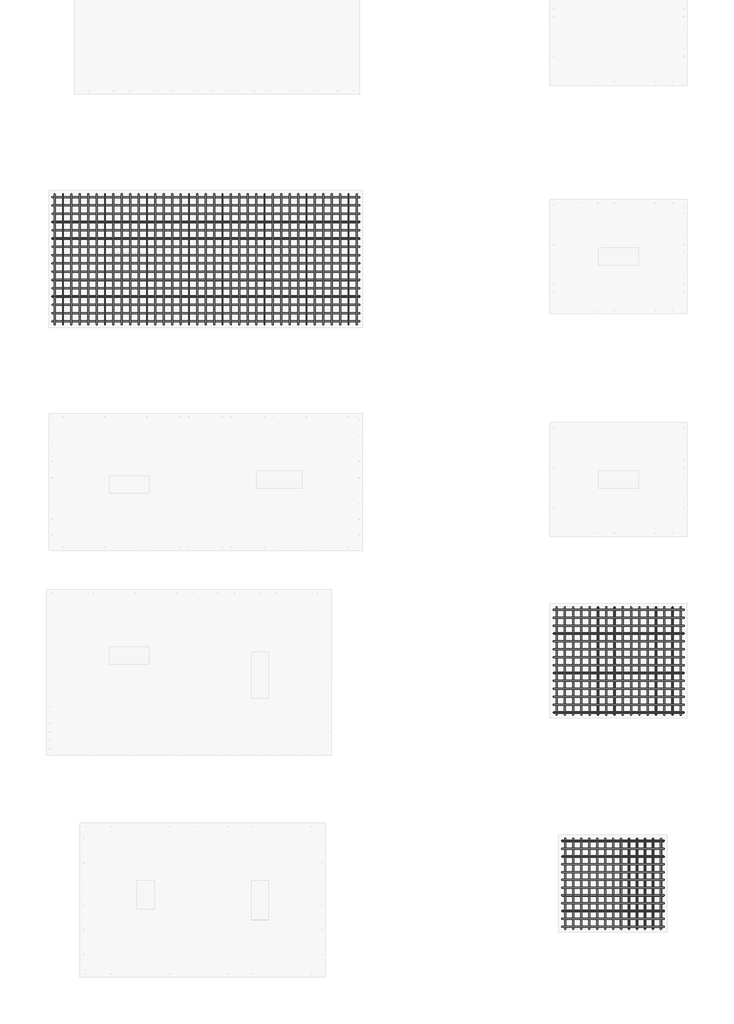
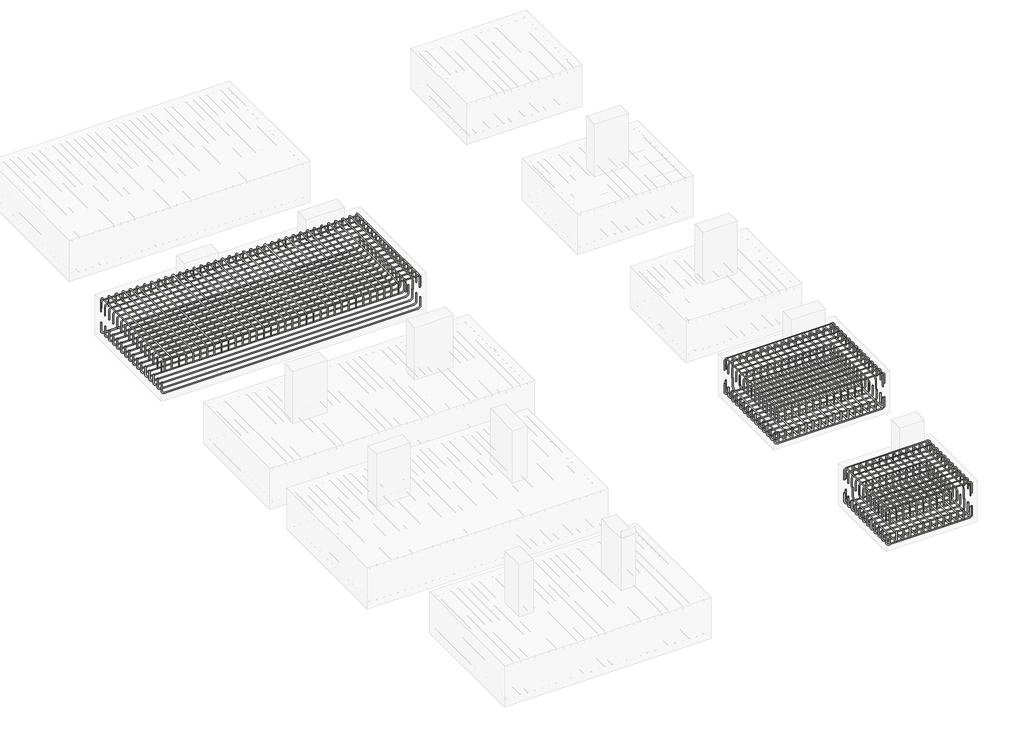
# One storey, part 8 of 21: 11 reinforcing bars.
"""IFC4 building model written with IfcOpenShell, lengths in millimetres."""

from ifc_helpers import new_model, si_unit, point, frame, origin, place, context, project, spatial, polyline, circle_curve, trimmed, segment, composite_curve, source, transform, mapped, element, save
from ifc_brep_helpers import swept_disk

model = new_model("IFC4")

# Units and contexts
model_context = context("Model", 3, world=origin())
ifc_project = project(units=[si_unit("LENGTHUNIT", "METRE", prefix="MILLI")], contexts=[model_context])

# Site, building, storey
site = spatial("IfcSite", under=ifc_project)
building = spatial("IfcBuilding", under=site)
storey = spatial("IfcBuildingStorey", under=building, Elevation=-1100.0)

# Reinforcing bars
placement = place(None, origin())
reinforcing_bar_shape = source(origin(), model_context, "Body", "SolidModel", [
    swept_disk(composite_curve([segment(polyline([(10485.4160849, -1642.8795712, -1400.0), (10485.4160849, -1642.8795712, -1213.4)]), True, "CONTINUOUS"), segment(trimmed(circle_curve(frame((10485.4160849, -1587.4295712, -1213.4), z_axis=(-1.0, 0.0, 0.0), x_axis=(0.0, -55.450000000000045, 0.0)), 55.45), [point((10485.4160849, -1642.8795712, -1213.4))], [point((10485.4160849, -1587.4295712, -1157.95))], True, "CARTESIAN"), True, "CONTINUOUS"), segment(polyline([(10485.4160849, -1587.4295712, -1157.95), (10485.4160849, 585.7704288, -1157.95)]), True, "CONTINUOUS"), segment(trimmed(circle_curve(frame((10485.4160849, 585.7704288, -1213.4), z_axis=(-1.0, 0.0, 0.0), x_axis=(0.0, 0.0, 55.450000000000045)), 55.45), [point((10485.4160849, 585.7704288, -1157.95))], [point((10485.4160849, 641.2204288, -1213.4))], True, "CARTESIAN"), True, "CONTINUOUS"), segment(polyline([(10485.4160849, 641.2204288, -1213.4), (10485.4160849, 641.2204288, -1400.0)]), True, "CONTINUOUS")], self_intersect=False), 7.95),
])
element("IfcReinforcingBar", 1, at=placement, inside=storey, context=model_context, shape_type="MappedRepresentation", body=[
    mapped(reinforcing_bar_shape, transform((0.0, 0.0, 0.0), x_axis=(1.0, 0.0, 0.0), y_axis=(0.0, 1.0, 0.0), z_axis=(0.0, 0.0, 1.0))),
    mapped(reinforcing_bar_shape, transform((147.2696553, 0.0, 0.0), x_axis=(1.0, 0.0, 0.0), y_axis=(0.0, 1.0, 0.0), z_axis=(0.0, 0.0, 1.0))),
    mapped(reinforcing_bar_shape, transform((294.5393106, 0.0, 0.0), x_axis=(1.0, 0.0, 0.0), y_axis=(0.0, 1.0, 0.0), z_axis=(0.0, 0.0, 1.0))),
    mapped(reinforcing_bar_shape, transform((441.8089659, 0.0, 0.0), x_axis=(1.0, 0.0, 0.0), y_axis=(0.0, 1.0, 0.0), z_axis=(0.0, 0.0, 1.0))),
    mapped(reinforcing_bar_shape, transform((589.0786213, 0.0, 0.0), x_axis=(1.0, 0.0, 0.0), y_axis=(0.0, 1.0, 0.0), z_axis=(0.0, 0.0, 1.0))),
    mapped(reinforcing_bar_shape, transform((736.3482766, 0.0, 0.0), x_axis=(1.0, 0.0, 0.0), y_axis=(0.0, 1.0, 0.0), z_axis=(0.0, 0.0, 1.0))),
    mapped(reinforcing_bar_shape, transform((883.6179319, 0.0, 0.0), x_axis=(1.0, 0.0, 0.0), y_axis=(0.0, 1.0, 0.0), z_axis=(0.0, 0.0, 1.0))),
    mapped(reinforcing_bar_shape, transform((1030.8875872, 0.0, 0.0), x_axis=(1.0, 0.0, 0.0), y_axis=(0.0, 1.0, 0.0), z_axis=(0.0, 0.0, 1.0))),
    mapped(reinforcing_bar_shape, transform((1178.1572425, 0.0, 0.0), x_axis=(1.0, 0.0, 0.0), y_axis=(0.0, 1.0, 0.0), z_axis=(0.0, 0.0, 1.0))),
    mapped(reinforcing_bar_shape, transform((1325.4268978, 0.0, 0.0), x_axis=(1.0, 0.0, 0.0), y_axis=(0.0, 1.0, 0.0), z_axis=(0.0, 0.0, 1.0))),
    mapped(reinforcing_bar_shape, transform((1472.6965532, 0.0, 0.0), x_axis=(1.0, 0.0, 0.0), y_axis=(0.0, 1.0, 0.0), z_axis=(0.0, 0.0, 1.0))),
    mapped(reinforcing_bar_shape, transform((1619.9662085, 0.0, 0.0), x_axis=(1.0, 0.0, 0.0), y_axis=(0.0, 1.0, 0.0), z_axis=(0.0, 0.0, 1.0))),
    mapped(reinforcing_bar_shape, transform((1767.2358638, 0.0, 0.0), x_axis=(1.0, 0.0, 0.0), y_axis=(0.0, 1.0, 0.0), z_axis=(0.0, 0.0, 1.0))),
    mapped(reinforcing_bar_shape, transform((1914.5055191, 0.0, 0.0), x_axis=(1.0, 0.0, 0.0), y_axis=(0.0, 1.0, 0.0), z_axis=(0.0, 0.0, 1.0))),
    mapped(reinforcing_bar_shape, transform((2061.7751744, 0.0, 0.0), x_axis=(1.0, 0.0, 0.0), y_axis=(0.0, 1.0, 0.0), z_axis=(0.0, 0.0, 1.0))),
    mapped(reinforcing_bar_shape, transform((2209.0448297, 0.0, 0.0), x_axis=(1.0, 0.0, 0.0), y_axis=(0.0, 1.0, 0.0), z_axis=(0.0, 0.0, 1.0))),
    mapped(reinforcing_bar_shape, transform((2356.314485, 0.0, 0.0), x_axis=(1.0, 0.0, 0.0), y_axis=(0.0, 1.0, 0.0), z_axis=(0.0, 0.0, 1.0))),
    mapped(reinforcing_bar_shape, transform((2503.5841404, 0.0, 0.0), x_axis=(1.0, 0.0, 0.0), y_axis=(0.0, 1.0, 0.0), z_axis=(0.0, 0.0, 1.0))),
    mapped(reinforcing_bar_shape, transform((2650.8537957, 0.0, 0.0), x_axis=(1.0, 0.0, 0.0), y_axis=(0.0, 1.0, 0.0), z_axis=(0.0, 0.0, 1.0))),
    mapped(reinforcing_bar_shape, transform((2798.123451, 0.0, 0.0), x_axis=(1.0, 0.0, 0.0), y_axis=(0.0, 1.0, 0.0), z_axis=(0.0, 0.0, 1.0))),
    mapped(reinforcing_bar_shape, transform((2945.3931063, 0.0, 0.0), x_axis=(1.0, 0.0, 0.0), y_axis=(0.0, 1.0, 0.0), z_axis=(0.0, 0.0, 1.0))),
    mapped(reinforcing_bar_shape, transform((3092.6627616, 0.0, 0.0), x_axis=(1.0, 0.0, 0.0), y_axis=(0.0, 1.0, 0.0), z_axis=(0.0, 0.0, 1.0))),
    mapped(reinforcing_bar_shape, transform((3239.9324169, 0.0, 0.0), x_axis=(1.0, 0.0, 0.0), y_axis=(0.0, 1.0, 0.0), z_axis=(0.0, 0.0, 1.0))),
    mapped(reinforcing_bar_shape, transform((3387.2020722, 0.0, 0.0), x_axis=(1.0, 0.0, 0.0), y_axis=(0.0, 1.0, 0.0), z_axis=(0.0, 0.0, 1.0))),
    mapped(reinforcing_bar_shape, transform((3534.4717276, 0.0, 0.0), x_axis=(1.0, 0.0, 0.0), y_axis=(0.0, 1.0, 0.0), z_axis=(0.0, 0.0, 1.0))),
    mapped(reinforcing_bar_shape, transform((3681.7413829, 0.0, 0.0), x_axis=(1.0, 0.0, 0.0), y_axis=(0.0, 1.0, 0.0), z_axis=(0.0, 0.0, 1.0))),
    mapped(reinforcing_bar_shape, transform((3829.0110382, 0.0, 0.0), x_axis=(1.0, 0.0, 0.0), y_axis=(0.0, 1.0, 0.0), z_axis=(0.0, 0.0, 1.0))),
    mapped(reinforcing_bar_shape, transform((3976.2806935, 0.0, 0.0), x_axis=(1.0, 0.0, 0.0), y_axis=(0.0, 1.0, 0.0), z_axis=(0.0, 0.0, 1.0))),
    mapped(reinforcing_bar_shape, transform((4123.5503488, 0.0, 0.0), x_axis=(1.0, 0.0, 0.0), y_axis=(0.0, 1.0, 0.0), z_axis=(0.0, 0.0, 1.0))),
    mapped(reinforcing_bar_shape, transform((4270.8200041, 0.0, 0.0), x_axis=(1.0, 0.0, 0.0), y_axis=(0.0, 1.0, 0.0), z_axis=(0.0, 0.0, 1.0))),
    mapped(reinforcing_bar_shape, transform((4418.0896595, 0.0, 0.0), x_axis=(1.0, 0.0, 0.0), y_axis=(0.0, 1.0, 0.0), z_axis=(0.0, 0.0, 1.0))),
    mapped(reinforcing_bar_shape, transform((4565.3593148, 0.0, 0.0), x_axis=(1.0, 0.0, 0.0), y_axis=(0.0, 1.0, 0.0), z_axis=(0.0, 0.0, 1.0))),
    mapped(reinforcing_bar_shape, transform((4712.6289701, 0.0, 0.0), x_axis=(1.0, 0.0, 0.0), y_axis=(0.0, 1.0, 0.0), z_axis=(0.0, 0.0, 1.0))),
    mapped(reinforcing_bar_shape, transform((4859.8986254, 0.0, 0.0), x_axis=(1.0, 0.0, 0.0), y_axis=(0.0, 1.0, 0.0), z_axis=(0.0, 0.0, 1.0))),
    mapped(reinforcing_bar_shape, transform((5007.1682807, 0.0, 0.0), x_axis=(1.0, 0.0, 0.0), y_axis=(0.0, 1.0, 0.0), z_axis=(0.0, 0.0, 1.0))),
    mapped(reinforcing_bar_shape, transform((5154.437936, 0.0, 0.0), x_axis=(1.0, 0.0, 0.0), y_axis=(0.0, 1.0, 0.0), z_axis=(0.0, 0.0, 1.0))),
    mapped(reinforcing_bar_shape, transform((5301.7075913, 0.0, 0.0), x_axis=(1.0, 0.0, 0.0), y_axis=(0.0, 1.0, 0.0), z_axis=(0.0, 0.0, 1.0))),
])
reinforcing_bar_2_shape = source(origin(), model_context, "Body", "SolidModel", [
    swept_disk(composite_curve([segment(polyline([(10447.1173137, 589.3862648, -1428.1111113), (10447.1173137, 589.3862648, -1241.5111113)]), True, "CONTINUOUS"), segment(trimmed(circle_curve(frame((10502.5673137, 589.3862648, -1241.5111113), z_axis=(0.0, 1.0, 0.0), x_axis=(-55.44999999999891, 0.0, 0.0)), 55.45), [point((10447.1173137, 589.3862648, -1241.5111113))], [point((10502.5673137, 589.3862648, -1186.0611113))], True, "CARTESIAN"), True, "CONTINUOUS"), segment(polyline([(10502.5673137, 589.3862648, -1186.0611113), (15775.7673137, 589.3862648, -1186.0611113)]), True, "CONTINUOUS"), segment(trimmed(circle_curve(frame((15775.7673137, 589.3862648, -1241.5111113), z_axis=(0.0, 1.0, 0.0), x_axis=(0.0, 0.0, 55.450000000000045)), 55.45), [point((15775.7673137, 589.3862648, -1186.0611113))], [point((15831.2173137, 589.3862648, -1241.5111113))], True, "CARTESIAN"), True, "CONTINUOUS"), segment(polyline([(15831.2173137, 589.3862648, -1241.5111113), (15831.2173137, 589.3862648, -1428.1111113)]), True, "CONTINUOUS")], self_intersect=False), 7.95),
])
element("IfcReinforcingBar", 2, at=placement, inside=storey, context=model_context, shape_type="MappedRepresentation", body=[
    mapped(reinforcing_bar_2_shape, transform((0.0, 0.0, 0.0), x_axis=(1.0, 0.0, 0.0), y_axis=(0.0, 1.0, 0.0), z_axis=(0.0, 0.0, 1.0))),
    mapped(reinforcing_bar_2_shape, transform((0.0, -145.2528929, 0.0), x_axis=(1.0, 0.0, 0.0), y_axis=(0.0, 1.0, 0.0), z_axis=(0.0, 0.0, 1.0))),
    mapped(reinforcing_bar_2_shape, transform((0.0, -290.5057858, 0.0), x_axis=(1.0, 0.0, 0.0), y_axis=(0.0, 1.0, 0.0), z_axis=(0.0, 0.0, 1.0))),
    mapped(reinforcing_bar_2_shape, transform((0.0, -435.7586787, 0.0), x_axis=(1.0, 0.0, 0.0), y_axis=(0.0, 1.0, 0.0), z_axis=(0.0, 0.0, 1.0))),
    mapped(reinforcing_bar_2_shape, transform((0.0, -581.0115716, 0.0), x_axis=(1.0, 0.0, 0.0), y_axis=(0.0, 1.0, 0.0), z_axis=(0.0, 0.0, 1.0))),
    mapped(reinforcing_bar_2_shape, transform((0.0, -726.2644645, 0.0), x_axis=(1.0, 0.0, 0.0), y_axis=(0.0, 1.0, 0.0), z_axis=(0.0, 0.0, 1.0))),
    mapped(reinforcing_bar_2_shape, transform((0.0, -871.5173574, 0.0), x_axis=(1.0, 0.0, 0.0), y_axis=(0.0, 1.0, 0.0), z_axis=(0.0, 0.0, 1.0))),
    mapped(reinforcing_bar_2_shape, transform((0.0, -1016.7702503, 0.0), x_axis=(1.0, 0.0, 0.0), y_axis=(0.0, 1.0, 0.0), z_axis=(0.0, 0.0, 1.0))),
    mapped(reinforcing_bar_2_shape, transform((0.0, -1162.0231432, 0.0), x_axis=(1.0, 0.0, 0.0), y_axis=(0.0, 1.0, 0.0), z_axis=(0.0, 0.0, 1.0))),
    mapped(reinforcing_bar_2_shape, transform((0.0, -1307.276036, 0.0), x_axis=(1.0, 0.0, 0.0), y_axis=(0.0, 1.0, 0.0), z_axis=(0.0, 0.0, 1.0))),
    mapped(reinforcing_bar_2_shape, transform((0.0, -1452.5289289, 0.0), x_axis=(1.0, 0.0, 0.0), y_axis=(0.0, 1.0, 0.0), z_axis=(0.0, 0.0, 1.0))),
    mapped(reinforcing_bar_2_shape, transform((0.0, -1597.7818218, 0.0), x_axis=(1.0, 0.0, 0.0), y_axis=(0.0, 1.0, 0.0), z_axis=(0.0, 0.0, 1.0))),
    mapped(reinforcing_bar_2_shape, transform((0.0, -1743.0347147, 0.0), x_axis=(1.0, 0.0, 0.0), y_axis=(0.0, 1.0, 0.0), z_axis=(0.0, 0.0, 1.0))),
    mapped(reinforcing_bar_2_shape, transform((0.0, -1888.2876076, 0.0), x_axis=(1.0, 0.0, 0.0), y_axis=(0.0, 1.0, 0.0), z_axis=(0.0, 0.0, 1.0))),
    mapped(reinforcing_bar_2_shape, transform((0.0, -2033.5405005, 0.0), x_axis=(1.0, 0.0, 0.0), y_axis=(0.0, 1.0, 0.0), z_axis=(0.0, 0.0, 1.0))),
    mapped(reinforcing_bar_2_shape, transform((0.0, -2178.7933934, 0.0), x_axis=(1.0, 0.0, 0.0), y_axis=(0.0, 1.0, 0.0), z_axis=(0.0, 0.0, 1.0))),
])
reinforcing_bar_3_shape = source(origin(), model_context, "Body", "SolidModel", [
    swept_disk(composite_curve([segment(polyline([(10449.1673137, -1589.4071286, -1669.8442859), (10449.1673137, -1589.4071286, -1852.3442859)]), True, "CONTINUOUS"), segment(trimmed(circle_curve(frame((10506.6673137, -1589.4071286, -1852.3442859), z_axis=(0.0, -1.0, 0.0), x_axis=(-57.5, 0.0, 0.0)), 57.5), [point((10449.1673137, -1589.4071286, -1852.3442859))], [point((10506.6673137, -1589.4071286, -1909.8442859))], True, "CARTESIAN"), True, "CONTINUOUS"), segment(polyline([(10506.6673137, -1589.4071286, -1909.8442859), (15771.6673137, -1589.4071286, -1909.8442859)]), True, "CONTINUOUS"), segment(trimmed(circle_curve(frame((15771.6673137, -1589.4071286, -1852.3442859), z_axis=(0.0, -1.0, 0.0), x_axis=(0.0, 0.0, -57.5)), 57.5), [point((15771.6673137, -1589.4071286, -1909.8442859))], [point((15829.1673137, -1589.4071286, -1852.3442859))], True, "CARTESIAN"), True, "CONTINUOUS"), segment(polyline([(15829.1673137, -1589.4071286, -1852.3442859), (15829.1673137, -1589.4071286, -1669.8442859)]), True, "CONTINUOUS")], self_intersect=False), 10.0),
])
element("IfcReinforcingBar", 3, at=placement, inside=storey, context=model_context, shape_type="MappedRepresentation", body=[
    mapped(reinforcing_bar_3_shape, transform((0.0, 0.0, 0.0), x_axis=(1.0, 0.0, 0.0), y_axis=(0.0, 1.0, 0.0), z_axis=(0.0, 0.0, 1.0))),
    mapped(reinforcing_bar_3_shape, transform((0.0, 145.2528929, 0.0), x_axis=(1.0, 0.0, 0.0), y_axis=(0.0, 1.0, 0.0), z_axis=(0.0, 0.0, 1.0))),
    mapped(reinforcing_bar_3_shape, transform((0.0, 290.5057858, 0.0), x_axis=(1.0, 0.0, 0.0), y_axis=(0.0, 1.0, 0.0), z_axis=(0.0, 0.0, 1.0))),
    mapped(reinforcing_bar_3_shape, transform((0.0, 435.7586787, 0.0), x_axis=(1.0, 0.0, 0.0), y_axis=(0.0, 1.0, 0.0), z_axis=(0.0, 0.0, 1.0))),
    mapped(reinforcing_bar_3_shape, transform((0.0, 581.0115716, 0.0), x_axis=(1.0, 0.0, 0.0), y_axis=(0.0, 1.0, 0.0), z_axis=(0.0, 0.0, 1.0))),
    mapped(reinforcing_bar_3_shape, transform((0.0, 726.2644645, 0.0), x_axis=(1.0, 0.0, 0.0), y_axis=(0.0, 1.0, 0.0), z_axis=(0.0, 0.0, 1.0))),
    mapped(reinforcing_bar_3_shape, transform((0.0, 871.5173574, 0.0), x_axis=(1.0, 0.0, 0.0), y_axis=(0.0, 1.0, 0.0), z_axis=(0.0, 0.0, 1.0))),
    mapped(reinforcing_bar_3_shape, transform((0.0, 1016.7702503, 0.0), x_axis=(1.0, 0.0, 0.0), y_axis=(0.0, 1.0, 0.0), z_axis=(0.0, 0.0, 1.0))),
    mapped(reinforcing_bar_3_shape, transform((0.0, 1162.0231432, 0.0), x_axis=(1.0, 0.0, 0.0), y_axis=(0.0, 1.0, 0.0), z_axis=(0.0, 0.0, 1.0))),
    mapped(reinforcing_bar_3_shape, transform((0.0, 1307.276036, 0.0), x_axis=(1.0, 0.0, 0.0), y_axis=(0.0, 1.0, 0.0), z_axis=(0.0, 0.0, 1.0))),
    mapped(reinforcing_bar_3_shape, transform((0.0, 1452.5289289, 0.0), x_axis=(1.0, 0.0, 0.0), y_axis=(0.0, 1.0, 0.0), z_axis=(0.0, 0.0, 1.0))),
    mapped(reinforcing_bar_3_shape, transform((0.0, 1597.7818218, 0.0), x_axis=(1.0, 0.0, 0.0), y_axis=(0.0, 1.0, 0.0), z_axis=(0.0, 0.0, 1.0))),
    mapped(reinforcing_bar_3_shape, transform((0.0, 1743.0347147, 0.0), x_axis=(1.0, 0.0, 0.0), y_axis=(0.0, 1.0, 0.0), z_axis=(0.0, 0.0, 1.0))),
    mapped(reinforcing_bar_3_shape, transform((0.0, 1888.2876076, 0.0), x_axis=(1.0, 0.0, 0.0), y_axis=(0.0, 1.0, 0.0), z_axis=(0.0, 0.0, 1.0))),
    mapped(reinforcing_bar_3_shape, transform((0.0, 2033.5405005, 0.0), x_axis=(1.0, 0.0, 0.0), y_axis=(0.0, 1.0, 0.0), z_axis=(0.0, 0.0, 1.0))),
    mapped(reinforcing_bar_3_shape, transform((0.0, 2178.7933934, 0.0), x_axis=(1.0, 0.0, 0.0), y_axis=(0.0, 1.0, 0.0), z_axis=(0.0, 0.0, 1.0))),
])
reinforcing_bar_4_shape = source(origin(), model_context, "Body", "SolidModel", [
    swept_disk(composite_curve([segment(polyline([(21169.1673137, -10702.0783425, -1700.0), (21169.1673137, -10702.0783425, -1882.5)]), True, "CONTINUOUS"), segment(trimmed(circle_curve(frame((21111.6673137, -10702.0783425, -1882.5), z_axis=(0.0, 1.0, 0.0), x_axis=(57.5, 0.0, 0.0)), 57.5), [point((21169.1673137, -10702.0783425, -1882.5))], [point((21111.6673137, -10702.0783425, -1940.0))], True, "CARTESIAN"), True, "CONTINUOUS"), segment(polyline([(21111.6673137, -10702.0783425, -1940.0), (19446.6673137, -10702.0783425, -1940.0)]), True, "CONTINUOUS"), segment(trimmed(circle_curve(frame((19446.6673137, -10702.0783425, -1882.5), z_axis=(0.0, 1.0, 0.0), x_axis=(0.0, 0.0, -57.5)), 57.5), [point((19446.6673137, -10702.0783425, -1940.0))], [point((19389.1673137, -10702.0783425, -1882.5))], True, "CARTESIAN"), True, "CONTINUOUS"), segment(polyline([(19389.1673137, -10702.0783425, -1882.5), (19389.1673137, -10702.0783425, -1700.0)]), True, "CONTINUOUS")], self_intersect=False), 10.0),
])
element("IfcReinforcingBar", 4, at=placement, inside=storey, context=model_context, shape_type="MappedRepresentation", body=[
    mapped(reinforcing_bar_4_shape, transform((0.0, 0.0, 0.0), x_axis=(1.0, 0.0, 0.0), y_axis=(0.0, 1.0, 0.0), z_axis=(0.0, 0.0, 1.0))),
    mapped(reinforcing_bar_4_shape, transform((0.0, -136.5188719, 0.0), x_axis=(1.0, 0.0, 0.0), y_axis=(0.0, 1.0, 0.0), z_axis=(0.0, 0.0, 1.0))),
    mapped(reinforcing_bar_4_shape, transform((0.0, -273.0377439, 0.0), x_axis=(1.0, 0.0, 0.0), y_axis=(0.0, 1.0, 0.0), z_axis=(0.0, 0.0, 1.0))),
    mapped(reinforcing_bar_4_shape, transform((0.0, -409.5566158, 0.0), x_axis=(1.0, 0.0, 0.0), y_axis=(0.0, 1.0, 0.0), z_axis=(0.0, 0.0, 1.0))),
    mapped(reinforcing_bar_4_shape, transform((0.0, -546.0754878, 0.0), x_axis=(1.0, 0.0, 0.0), y_axis=(0.0, 1.0, 0.0), z_axis=(0.0, 0.0, 1.0))),
    mapped(reinforcing_bar_4_shape, transform((0.0, -682.5943597, 0.0), x_axis=(1.0, 0.0, 0.0), y_axis=(0.0, 1.0, 0.0), z_axis=(0.0, 0.0, 1.0))),
    mapped(reinforcing_bar_4_shape, transform((0.0, -819.1132316, 0.0), x_axis=(1.0, 0.0, 0.0), y_axis=(0.0, 1.0, 0.0), z_axis=(0.0, 0.0, 1.0))),
    mapped(reinforcing_bar_4_shape, transform((0.0, -955.6321036, 0.0), x_axis=(1.0, 0.0, 0.0), y_axis=(0.0, 1.0, 0.0), z_axis=(0.0, 0.0, 1.0))),
    mapped(reinforcing_bar_4_shape, transform((0.0, -1092.1509755, 0.0), x_axis=(1.0, 0.0, 0.0), y_axis=(0.0, 1.0, 0.0), z_axis=(0.0, 0.0, 1.0))),
    mapped(reinforcing_bar_4_shape, transform((0.0, -1228.6698475, 0.0), x_axis=(1.0, 0.0, 0.0), y_axis=(0.0, 1.0, 0.0), z_axis=(0.0, 0.0, 1.0))),
    mapped(reinforcing_bar_4_shape, transform((0.0, -1365.1887194, 0.0), x_axis=(1.0, 0.0, 0.0), y_axis=(0.0, 1.0, 0.0), z_axis=(0.0, 0.0, 1.0))),
    mapped(reinforcing_bar_4_shape, transform((0.0, -1501.7075913, 0.0), x_axis=(1.0, 0.0, 0.0), y_axis=(0.0, 1.0, 0.0), z_axis=(0.0, 0.0, 1.0))),
])
reinforcing_bar_5_shape = source(origin(), model_context, "Body", "SolidModel", [
    swept_disk(composite_curve([segment(polyline([(19387.1173137, -10702.0783425, -1400.0), (19387.1173137, -10702.0783425, -1213.4)]), True, "CONTINUOUS"), segment(trimmed(circle_curve(frame((19442.5673137, -10702.0783425, -1213.4), z_axis=(0.0, 1.0, 0.0), x_axis=(-55.45000000000073, 0.0, 0.0)), 55.45), [point((19387.1173137, -10702.0783425, -1213.4))], [point((19442.5673137, -10702.0783425, -1157.95))], True, "CARTESIAN"), True, "CONTINUOUS"), segment(polyline([(19442.5673137, -10702.0783425, -1157.95), (21115.7673137, -10702.0783425, -1157.95)]), True, "CONTINUOUS"), segment(trimmed(circle_curve(frame((21115.7673137, -10702.0783425, -1213.4), z_axis=(0.0, 1.0, 0.0), x_axis=(0.0, 0.0, 55.450000000000045)), 55.45), [point((21115.7673137, -10702.0783425, -1157.95))], [point((21171.2173137, -10702.0783425, -1213.4))], True, "CARTESIAN"), True, "CONTINUOUS"), segment(polyline([(21171.2173137, -10702.0783425, -1213.4), (21171.2173137, -10702.0783425, -1400.0)]), True, "CONTINUOUS")], self_intersect=False), 7.95),
])
element("IfcReinforcingBar", 5, at=placement, inside=storey, context=model_context, shape_type="MappedRepresentation", body=[
    mapped(reinforcing_bar_5_shape, transform((0.0, 0.0, 0.0), x_axis=(1.0, 0.0, 0.0), y_axis=(0.0, 1.0, 0.0), z_axis=(0.0, 0.0, 1.0))),
    mapped(reinforcing_bar_5_shape, transform((0.0, -136.5188719, 0.0), x_axis=(1.0, 0.0, 0.0), y_axis=(0.0, 1.0, 0.0), z_axis=(0.0, 0.0, 1.0))),
    mapped(reinforcing_bar_5_shape, transform((0.0, -273.0377439, 0.0), x_axis=(1.0, 0.0, 0.0), y_axis=(0.0, 1.0, 0.0), z_axis=(0.0, 0.0, 1.0))),
    mapped(reinforcing_bar_5_shape, transform((0.0, -409.5566158, 0.0), x_axis=(1.0, 0.0, 0.0), y_axis=(0.0, 1.0, 0.0), z_axis=(0.0, 0.0, 1.0))),
    mapped(reinforcing_bar_5_shape, transform((0.0, -546.0754878, 0.0), x_axis=(1.0, 0.0, 0.0), y_axis=(0.0, 1.0, 0.0), z_axis=(0.0, 0.0, 1.0))),
    mapped(reinforcing_bar_5_shape, transform((0.0, -682.5943597, 0.0), x_axis=(1.0, 0.0, 0.0), y_axis=(0.0, 1.0, 0.0), z_axis=(0.0, 0.0, 1.0))),
    mapped(reinforcing_bar_5_shape, transform((0.0, -819.1132316, 0.0), x_axis=(1.0, 0.0, 0.0), y_axis=(0.0, 1.0, 0.0), z_axis=(0.0, 0.0, 1.0))),
    mapped(reinforcing_bar_5_shape, transform((0.0, -955.6321036, 0.0), x_axis=(1.0, 0.0, 0.0), y_axis=(0.0, 1.0, 0.0), z_axis=(0.0, 0.0, 1.0))),
    mapped(reinforcing_bar_5_shape, transform((0.0, -1092.1509755, 0.0), x_axis=(1.0, 0.0, 0.0), y_axis=(0.0, 1.0, 0.0), z_axis=(0.0, 0.0, 1.0))),
    mapped(reinforcing_bar_5_shape, transform((0.0, -1228.6698475, 0.0), x_axis=(1.0, 0.0, 0.0), y_axis=(0.0, 1.0, 0.0), z_axis=(0.0, 0.0, 1.0))),
    mapped(reinforcing_bar_5_shape, transform((0.0, -1365.1887194, 0.0), x_axis=(1.0, 0.0, 0.0), y_axis=(0.0, 1.0, 0.0), z_axis=(0.0, 0.0, 1.0))),
    mapped(reinforcing_bar_5_shape, transform((0.0, -1501.7075913, 0.0), x_axis=(1.0, 0.0, 0.0), y_axis=(0.0, 1.0, 0.0), z_axis=(0.0, 0.0, 1.0))),
])
reinforcing_bar_6_shape = source(origin(), model_context, "Body", "SolidModel", [
    swept_disk(composite_curve([segment(polyline([(21119.3831496, -10663.7795712, -1428.1111113), (21119.3831496, -10663.7795712, -1241.5111113)]), True, "CONTINUOUS"), segment(trimmed(circle_curve(frame((21119.3831496, -10719.2295712, -1241.5111113), z_axis=(1.0, 0.0, 0.0), x_axis=(0.0, 55.44999999999891, 0.0)), 55.45), [point((21119.3831496, -10663.7795712, -1241.5111113))], [point((21119.3831496, -10719.2295712, -1186.0611113))], True, "CARTESIAN"), True, "CONTINUOUS"), segment(polyline([(21119.3831496, -10719.2295712, -1186.0611113), (21119.3831496, -12192.4295712, -1186.0611113)]), True, "CONTINUOUS"), segment(trimmed(circle_curve(frame((21119.3831496, -12192.4295712, -1241.5111113), z_axis=(1.0, 0.0, 0.0), x_axis=(0.0, 0.0, 55.450000000000045)), 55.45), [point((21119.3831496, -12192.4295712, -1186.0611113))], [point((21119.3831496, -12247.8795712, -1241.5111113))], True, "CARTESIAN"), True, "CONTINUOUS"), segment(polyline([(21119.3831496, -12247.8795712, -1241.5111113), (21119.3831496, -12247.8795712, -1428.1111113)]), True, "CONTINUOUS")], self_intersect=False), 7.95),
])
element("IfcReinforcingBar", 6, at=placement, inside=storey, context=model_context, shape_type="MappedRepresentation", body=[
    mapped(reinforcing_bar_6_shape, transform((0.0, 0.0, 0.0), x_axis=(1.0, 0.0, 0.0), y_axis=(0.0, 1.0, 0.0), z_axis=(0.0, 0.0, 1.0))),
    mapped(reinforcing_bar_6_shape, transform((-139.8994495, 0.0, 0.0), x_axis=(1.0, 0.0, 0.0), y_axis=(0.0, 1.0, 0.0), z_axis=(0.0, 0.0, 1.0))),
    mapped(reinforcing_bar_6_shape, transform((-279.7988989, 0.0, 0.0), x_axis=(1.0, 0.0, 0.0), y_axis=(0.0, 1.0, 0.0), z_axis=(0.0, 0.0, 1.0))),
    mapped(reinforcing_bar_6_shape, transform((-419.6983484, 0.0, 0.0), x_axis=(1.0, 0.0, 0.0), y_axis=(0.0, 1.0, 0.0), z_axis=(0.0, 0.0, 1.0))),
    mapped(reinforcing_bar_6_shape, transform((-559.5977978, 0.0, 0.0), x_axis=(1.0, 0.0, 0.0), y_axis=(0.0, 1.0, 0.0), z_axis=(0.0, 0.0, 1.0))),
    mapped(reinforcing_bar_6_shape, transform((-699.4972473, 0.0, 0.0), x_axis=(1.0, 0.0, 0.0), y_axis=(0.0, 1.0, 0.0), z_axis=(0.0, 0.0, 1.0))),
    mapped(reinforcing_bar_6_shape, transform((-839.3966967, 0.0, 0.0), x_axis=(1.0, 0.0, 0.0), y_axis=(0.0, 1.0, 0.0), z_axis=(0.0, 0.0, 1.0))),
    mapped(reinforcing_bar_6_shape, transform((-979.2961462, 0.0, 0.0), x_axis=(1.0, 0.0, 0.0), y_axis=(0.0, 1.0, 0.0), z_axis=(0.0, 0.0, 1.0))),
    mapped(reinforcing_bar_6_shape, transform((-1119.1955956, 0.0, 0.0), x_axis=(1.0, 0.0, 0.0), y_axis=(0.0, 1.0, 0.0), z_axis=(0.0, 0.0, 1.0))),
    mapped(reinforcing_bar_6_shape, transform((-1259.0950451, 0.0, 0.0), x_axis=(1.0, 0.0, 0.0), y_axis=(0.0, 1.0, 0.0), z_axis=(0.0, 0.0, 1.0))),
    mapped(reinforcing_bar_6_shape, transform((-1398.9944945, 0.0, 0.0), x_axis=(1.0, 0.0, 0.0), y_axis=(0.0, 1.0, 0.0), z_axis=(0.0, 0.0, 1.0))),
    mapped(reinforcing_bar_6_shape, transform((-1538.893944, 0.0, 0.0), x_axis=(1.0, 0.0, 0.0), y_axis=(0.0, 1.0, 0.0), z_axis=(0.0, 0.0, 1.0))),
    mapped(reinforcing_bar_6_shape, transform((-1678.7933934, 0.0, 0.0), x_axis=(1.0, 0.0, 0.0), y_axis=(0.0, 1.0, 0.0), z_axis=(0.0, 0.0, 1.0))),
])
reinforcing_bar_7_shape = source(origin(), model_context, "Body", "SolidModel", [
    swept_disk(composite_curve([segment(polyline([(19440.5897562, -10665.8295712, -1669.8442859), (19440.5897562, -10665.8295712, -1852.3442859)]), True, "CONTINUOUS"), segment(trimmed(circle_curve(frame((19440.5897562, -10723.3295712, -1852.3442859), z_axis=(-1.0, 0.0, 0.0), x_axis=(0.0, 57.5, 0.0)), 57.5), [point((19440.5897562, -10665.8295712, -1852.3442859))], [point((19440.5897562, -10723.3295712, -1909.8442859))], True, "CARTESIAN"), True, "CONTINUOUS"), segment(polyline([(19440.5897562, -10723.3295712, -1909.8442859), (19440.5897562, -12188.3295712, -1909.8442859)]), True, "CONTINUOUS"), segment(trimmed(circle_curve(frame((19440.5897562, -12188.3295712, -1852.3442859), z_axis=(-1.0, 0.0, 0.0), x_axis=(0.0, 0.0, -57.5)), 57.5), [point((19440.5897562, -12188.3295712, -1909.8442859))], [point((19440.5897562, -12245.8295712, -1852.3442859))], True, "CARTESIAN"), True, "CONTINUOUS"), segment(polyline([(19440.5897562, -12245.8295712, -1852.3442859), (19440.5897562, -12245.8295712, -1669.8442859)]), True, "CONTINUOUS")], self_intersect=False), 10.0),
])
element("IfcReinforcingBar", 7, at=placement, inside=storey, context=model_context, shape_type="MappedRepresentation", body=[
    mapped(reinforcing_bar_7_shape, transform((0.0, 0.0, 0.0), x_axis=(1.0, 0.0, 0.0), y_axis=(0.0, 1.0, 0.0), z_axis=(0.0, 0.0, 1.0))),
    mapped(reinforcing_bar_7_shape, transform((139.8994495, 0.0, 0.0), x_axis=(1.0, 0.0, 0.0), y_axis=(0.0, 1.0, 0.0), z_axis=(0.0, 0.0, 1.0))),
    mapped(reinforcing_bar_7_shape, transform((279.7988989, 0.0, 0.0), x_axis=(1.0, 0.0, 0.0), y_axis=(0.0, 1.0, 0.0), z_axis=(0.0, 0.0, 1.0))),
    mapped(reinforcing_bar_7_shape, transform((419.6983484, 0.0, 0.0), x_axis=(1.0, 0.0, 0.0), y_axis=(0.0, 1.0, 0.0), z_axis=(0.0, 0.0, 1.0))),
    mapped(reinforcing_bar_7_shape, transform((559.5977978, 0.0, 0.0), x_axis=(1.0, 0.0, 0.0), y_axis=(0.0, 1.0, 0.0), z_axis=(0.0, 0.0, 1.0))),
    mapped(reinforcing_bar_7_shape, transform((699.4972473, 0.0, 0.0), x_axis=(1.0, 0.0, 0.0), y_axis=(0.0, 1.0, 0.0), z_axis=(0.0, 0.0, 1.0))),
    mapped(reinforcing_bar_7_shape, transform((839.3966967, 0.0, 0.0), x_axis=(1.0, 0.0, 0.0), y_axis=(0.0, 1.0, 0.0), z_axis=(0.0, 0.0, 1.0))),
    mapped(reinforcing_bar_7_shape, transform((979.2961462, 0.0, 0.0), x_axis=(1.0, 0.0, 0.0), y_axis=(0.0, 1.0, 0.0), z_axis=(0.0, 0.0, 1.0))),
    mapped(reinforcing_bar_7_shape, transform((1119.1955956, 0.0, 0.0), x_axis=(1.0, 0.0, 0.0), y_axis=(0.0, 1.0, 0.0), z_axis=(0.0, 0.0, 1.0))),
    mapped(reinforcing_bar_7_shape, transform((1259.0950451, 0.0, 0.0), x_axis=(1.0, 0.0, 0.0), y_axis=(0.0, 1.0, 0.0), z_axis=(0.0, 0.0, 1.0))),
    mapped(reinforcing_bar_7_shape, transform((1398.9944945, 0.0, 0.0), x_axis=(1.0, 0.0, 0.0), y_axis=(0.0, 1.0, 0.0), z_axis=(0.0, 0.0, 1.0))),
    mapped(reinforcing_bar_7_shape, transform((1538.893944, 0.0, 0.0), x_axis=(1.0, 0.0, 0.0), y_axis=(0.0, 1.0, 0.0), z_axis=(0.0, 0.0, 1.0))),
    mapped(reinforcing_bar_7_shape, transform((1678.7933934, 0.0, 0.0), x_axis=(1.0, 0.0, 0.0), y_axis=(0.0, 1.0, 0.0), z_axis=(0.0, 0.0, 1.0))),
])
reinforcing_bar_8_shape = source(origin(), model_context, "Body", "SolidModel", [
    swept_disk(composite_curve([segment(polyline([(19239.1673659, -8449.5807999, -1700.0), (19239.1673659, -8449.5807999, -1882.5)]), True, "CONTINUOUS"), segment(trimmed(circle_curve(frame((19296.6673659, -8449.5807999, -1882.5), z_axis=(0.0, -1.0, 0.0), x_axis=(-57.5, 0.0, 0.0)), 57.5), [point((19239.1673659, -8449.5807999, -1882.5))], [point((19296.6673659, -8449.5807999, -1940.0))], True, "CARTESIAN"), True, "CONTINUOUS"), segment(polyline([(19296.6673659, -8449.5807999, -1940.0), (21461.6673659, -8449.5807999, -1940.0)]), True, "CONTINUOUS"), segment(trimmed(circle_curve(frame((21461.6673659, -8449.5807999, -1882.5), z_axis=(0.0, -1.0, 0.0), x_axis=(0.0, 0.0, -57.5)), 57.5), [point((21461.6673659, -8449.5807999, -1940.0))], [point((21519.1673659, -8449.5807999, -1882.5))], True, "CARTESIAN"), True, "CONTINUOUS"), segment(polyline([(21519.1673659, -8449.5807999, -1882.5), (21519.1673659, -8449.5807999, -1700.0)]), True, "CONTINUOUS")], self_intersect=False), 10.0),
])
element("IfcReinforcingBar", 8, at=placement, inside=storey, context=model_context, shape_type="MappedRepresentation", body=[
    mapped(reinforcing_bar_8_shape, transform((0.0, 0.0, 0.0), x_axis=(1.0, 0.0, 0.0), y_axis=(0.0, 1.0, 0.0), z_axis=(0.0, 0.0, 1.0))),
    mapped(reinforcing_bar_8_shape, transform((0.0, 138.5928916, 0.0), x_axis=(1.0, 0.0, 0.0), y_axis=(0.0, 1.0, 0.0), z_axis=(0.0, 0.0, 1.0))),
    mapped(reinforcing_bar_8_shape, transform((0.0, 277.1857833, 0.0), x_axis=(1.0, 0.0, 0.0), y_axis=(0.0, 1.0, 0.0), z_axis=(0.0, 0.0, 1.0))),
    mapped(reinforcing_bar_8_shape, transform((0.0, 415.7786749, 0.0), x_axis=(1.0, 0.0, 0.0), y_axis=(0.0, 1.0, 0.0), z_axis=(0.0, 0.0, 1.0))),
    mapped(reinforcing_bar_8_shape, transform((0.0, 554.3715666, 0.0), x_axis=(1.0, 0.0, 0.0), y_axis=(0.0, 1.0, 0.0), z_axis=(0.0, 0.0, 1.0))),
    mapped(reinforcing_bar_8_shape, transform((0.0, 692.9644582, 0.0), x_axis=(1.0, 0.0, 0.0), y_axis=(0.0, 1.0, 0.0), z_axis=(0.0, 0.0, 1.0))),
    mapped(reinforcing_bar_8_shape, transform((0.0, 831.5573499, 0.0), x_axis=(1.0, 0.0, 0.0), y_axis=(0.0, 1.0, 0.0), z_axis=(0.0, 0.0, 1.0))),
    mapped(reinforcing_bar_8_shape, transform((0.0, 970.1502415, 0.0), x_axis=(1.0, 0.0, 0.0), y_axis=(0.0, 1.0, 0.0), z_axis=(0.0, 0.0, 1.0))),
    mapped(reinforcing_bar_8_shape, transform((0.0, 1108.7431331, 0.0), x_axis=(1.0, 0.0, 0.0), y_axis=(0.0, 1.0, 0.0), z_axis=(0.0, 0.0, 1.0))),
    mapped(reinforcing_bar_8_shape, transform((0.0, 1247.3360248, 0.0), x_axis=(1.0, 0.0, 0.0), y_axis=(0.0, 1.0, 0.0), z_axis=(0.0, 0.0, 1.0))),
    mapped(reinforcing_bar_8_shape, transform((0.0, 1385.9289164, 0.0), x_axis=(1.0, 0.0, 0.0), y_axis=(0.0, 1.0, 0.0), z_axis=(0.0, 0.0, 1.0))),
    mapped(reinforcing_bar_8_shape, transform((0.0, 1524.5218081, 0.0), x_axis=(1.0, 0.0, 0.0), y_axis=(0.0, 1.0, 0.0), z_axis=(0.0, 0.0, 1.0))),
    mapped(reinforcing_bar_8_shape, transform((0.0, 1663.1146997, 0.0), x_axis=(1.0, 0.0, 0.0), y_axis=(0.0, 1.0, 0.0), z_axis=(0.0, 0.0, 1.0))),
    mapped(reinforcing_bar_8_shape, transform((0.0, 1801.7075913, 0.0), x_axis=(1.0, 0.0, 0.0), y_axis=(0.0, 1.0, 0.0), z_axis=(0.0, 0.0, 1.0))),
])
reinforcing_bar_9_shape = source(origin(), model_context, "Body", "SolidModel", [
    swept_disk(composite_curve([segment(polyline([(21521.2173659, -8449.5807999, -1400.0), (21521.2173659, -8449.5807999, -1213.4)]), True, "CONTINUOUS"), segment(trimmed(circle_curve(frame((21465.7673659, -8449.5807999, -1213.4), z_axis=(0.0, -1.0, 0.0), x_axis=(55.45000000000073, 0.0, 0.0)), 55.45), [point((21521.2173659, -8449.5807999, -1213.4))], [point((21465.7673659, -8449.5807999, -1157.95))], True, "CARTESIAN"), True, "CONTINUOUS"), segment(polyline([(21465.7673659, -8449.5807999, -1157.95), (19292.5673659, -8449.5807999, -1157.95)]), True, "CONTINUOUS"), segment(trimmed(circle_curve(frame((19292.5673659, -8449.5807999, -1213.4), z_axis=(0.0, -1.0, 0.0), x_axis=(0.0, 0.0, 55.450000000000045)), 55.45), [point((19292.5673659, -8449.5807999, -1157.95))], [point((19237.1173659, -8449.5807999, -1213.4))], True, "CARTESIAN"), True, "CONTINUOUS"), segment(polyline([(19237.1173659, -8449.5807999, -1213.4), (19237.1173659, -8449.5807999, -1400.0)]), True, "CONTINUOUS")], self_intersect=False), 7.95),
])
element("IfcReinforcingBar", 9, at=placement, inside=storey, context=model_context, shape_type="MappedRepresentation", body=[
    mapped(reinforcing_bar_9_shape, transform((0.0, 0.0, 0.0), x_axis=(1.0, 0.0, 0.0), y_axis=(0.0, 1.0, 0.0), z_axis=(0.0, 0.0, 1.0))),
    mapped(reinforcing_bar_9_shape, transform((0.0, 138.5928916, 0.0), x_axis=(1.0, 0.0, 0.0), y_axis=(0.0, 1.0, 0.0), z_axis=(0.0, 0.0, 1.0))),
    mapped(reinforcing_bar_9_shape, transform((0.0, 277.1857833, 0.0), x_axis=(1.0, 0.0, 0.0), y_axis=(0.0, 1.0, 0.0), z_axis=(0.0, 0.0, 1.0))),
    mapped(reinforcing_bar_9_shape, transform((0.0, 415.7786749, 0.0), x_axis=(1.0, 0.0, 0.0), y_axis=(0.0, 1.0, 0.0), z_axis=(0.0, 0.0, 1.0))),
    mapped(reinforcing_bar_9_shape, transform((0.0, 554.3715666, 0.0), x_axis=(1.0, 0.0, 0.0), y_axis=(0.0, 1.0, 0.0), z_axis=(0.0, 0.0, 1.0))),
    mapped(reinforcing_bar_9_shape, transform((0.0, 692.9644582, 0.0), x_axis=(1.0, 0.0, 0.0), y_axis=(0.0, 1.0, 0.0), z_axis=(0.0, 0.0, 1.0))),
    mapped(reinforcing_bar_9_shape, transform((0.0, 831.5573499, 0.0), x_axis=(1.0, 0.0, 0.0), y_axis=(0.0, 1.0, 0.0), z_axis=(0.0, 0.0, 1.0))),
    mapped(reinforcing_bar_9_shape, transform((0.0, 970.1502415, 0.0), x_axis=(1.0, 0.0, 0.0), y_axis=(0.0, 1.0, 0.0), z_axis=(0.0, 0.0, 1.0))),
    mapped(reinforcing_bar_9_shape, transform((0.0, 1108.7431331, 0.0), x_axis=(1.0, 0.0, 0.0), y_axis=(0.0, 1.0, 0.0), z_axis=(0.0, 0.0, 1.0))),
    mapped(reinforcing_bar_9_shape, transform((0.0, 1247.3360248, 0.0), x_axis=(1.0, 0.0, 0.0), y_axis=(0.0, 1.0, 0.0), z_axis=(0.0, 0.0, 1.0))),
    mapped(reinforcing_bar_9_shape, transform((0.0, 1385.9289164, 0.0), x_axis=(1.0, 0.0, 0.0), y_axis=(0.0, 1.0, 0.0), z_axis=(0.0, 0.0, 1.0))),
    mapped(reinforcing_bar_9_shape, transform((0.0, 1524.5218081, 0.0), x_axis=(1.0, 0.0, 0.0), y_axis=(0.0, 1.0, 0.0), z_axis=(0.0, 0.0, 1.0))),
    mapped(reinforcing_bar_9_shape, transform((0.0, 1663.1146997, 0.0), x_axis=(1.0, 0.0, 0.0), y_axis=(0.0, 1.0, 0.0), z_axis=(0.0, 0.0, 1.0))),
    mapped(reinforcing_bar_9_shape, transform((0.0, 1801.7075913, 0.0), x_axis=(1.0, 0.0, 0.0), y_axis=(0.0, 1.0, 0.0), z_axis=(0.0, 0.0, 1.0))),
])
reinforcing_bar_10_shape = source(origin(), model_context, "Body", "SolidModel", [
    swept_disk(composite_curve([segment(polyline([(19288.9515299, -8487.8795712, -1428.1111113), (19288.9515299, -8487.8795712, -1241.5111113)]), True, "CONTINUOUS"), segment(trimmed(circle_curve(frame((19288.9515299, -8432.4295712, -1241.5111113), z_axis=(-1.0, 0.0, 0.0), x_axis=(0.0, -55.44999999999891, 0.0)), 55.45), [point((19288.9515299, -8487.8795712, -1241.5111113))], [point((19288.9515299, -8432.4295712, -1186.0611113))], True, "CARTESIAN"), True, "CONTINUOUS"), segment(polyline([(19288.9515299, -8432.4295712, -1186.0611113), (19288.9515299, -6659.2295712, -1186.0611113)]), True, "CONTINUOUS"), segment(trimmed(circle_curve(frame((19288.9515299, -6659.2295712, -1241.5111113), z_axis=(-1.0, 0.0, 0.0), x_axis=(0.0, 0.0, 55.450000000000045)), 55.45), [point((19288.9515299, -6659.2295712, -1186.0611113))], [point((19288.9515299, -6603.7795712, -1241.5111113))], True, "CARTESIAN"), True, "CONTINUOUS"), segment(polyline([(19288.9515299, -6603.7795712, -1241.5111113), (19288.9515299, -6603.7795712, -1428.1111113)]), True, "CONTINUOUS")], self_intersect=False), 7.95),
])
element("IfcReinforcingBar", 10, at=placement, inside=storey, context=model_context, shape_type="MappedRepresentation", body=[
    mapped(reinforcing_bar_10_shape, transform((0.0, 0.0, 0.0), x_axis=(1.0, 0.0, 0.0), y_axis=(0.0, 1.0, 0.0), z_axis=(0.0, 0.0, 1.0))),
    mapped(reinforcing_bar_10_shape, transform((145.2528929, 0.0, 0.0), x_axis=(1.0, 0.0, 0.0), y_axis=(0.0, 1.0, 0.0), z_axis=(0.0, 0.0, 1.0))),
    mapped(reinforcing_bar_10_shape, transform((290.5057858, 0.0, 0.0), x_axis=(1.0, 0.0, 0.0), y_axis=(0.0, 1.0, 0.0), z_axis=(0.0, 0.0, 1.0))),
    mapped(reinforcing_bar_10_shape, transform((435.7586787, 0.0, 0.0), x_axis=(1.0, 0.0, 0.0), y_axis=(0.0, 1.0, 0.0), z_axis=(0.0, 0.0, 1.0))),
    mapped(reinforcing_bar_10_shape, transform((581.0115716, 0.0, 0.0), x_axis=(1.0, 0.0, 0.0), y_axis=(0.0, 1.0, 0.0), z_axis=(0.0, 0.0, 1.0))),
    mapped(reinforcing_bar_10_shape, transform((726.2644645, 0.0, 0.0), x_axis=(1.0, 0.0, 0.0), y_axis=(0.0, 1.0, 0.0), z_axis=(0.0, 0.0, 1.0))),
    mapped(reinforcing_bar_10_shape, transform((871.5173574, 0.0, 0.0), x_axis=(1.0, 0.0, 0.0), y_axis=(0.0, 1.0, 0.0), z_axis=(0.0, 0.0, 1.0))),
    mapped(reinforcing_bar_10_shape, transform((1016.7702503, 0.0, 0.0), x_axis=(1.0, 0.0, 0.0), y_axis=(0.0, 1.0, 0.0), z_axis=(0.0, 0.0, 1.0))),
    mapped(reinforcing_bar_10_shape, transform((1162.0231432, 0.0, 0.0), x_axis=(1.0, 0.0, 0.0), y_axis=(0.0, 1.0, 0.0), z_axis=(0.0, 0.0, 1.0))),
    mapped(reinforcing_bar_10_shape, transform((1307.276036, 0.0, 0.0), x_axis=(1.0, 0.0, 0.0), y_axis=(0.0, 1.0, 0.0), z_axis=(0.0, 0.0, 1.0))),
    mapped(reinforcing_bar_10_shape, transform((1452.5289289, 0.0, 0.0), x_axis=(1.0, 0.0, 0.0), y_axis=(0.0, 1.0, 0.0), z_axis=(0.0, 0.0, 1.0))),
    mapped(reinforcing_bar_10_shape, transform((1597.7818218, 0.0, 0.0), x_axis=(1.0, 0.0, 0.0), y_axis=(0.0, 1.0, 0.0), z_axis=(0.0, 0.0, 1.0))),
    mapped(reinforcing_bar_10_shape, transform((1743.0347147, 0.0, 0.0), x_axis=(1.0, 0.0, 0.0), y_axis=(0.0, 1.0, 0.0), z_axis=(0.0, 0.0, 1.0))),
    mapped(reinforcing_bar_10_shape, transform((1888.2876076, 0.0, 0.0), x_axis=(1.0, 0.0, 0.0), y_axis=(0.0, 1.0, 0.0), z_axis=(0.0, 0.0, 1.0))),
    mapped(reinforcing_bar_10_shape, transform((2033.5405005, 0.0, 0.0), x_axis=(1.0, 0.0, 0.0), y_axis=(0.0, 1.0, 0.0), z_axis=(0.0, 0.0, 1.0))),
    mapped(reinforcing_bar_10_shape, transform((2178.7933934, 0.0, 0.0), x_axis=(1.0, 0.0, 0.0), y_axis=(0.0, 1.0, 0.0), z_axis=(0.0, 0.0, 1.0))),
])
reinforcing_bar_11_shape = source(origin(), model_context, "Body", "SolidModel", [
    swept_disk(composite_curve([segment(polyline([(21467.7449233, -8485.8295712, -1669.8442859), (21467.7449233, -8485.8295712, -1852.3442859)]), True, "CONTINUOUS"), segment(trimmed(circle_curve(frame((21467.7449233, -8428.3295712, -1852.3442859), z_axis=(1.0, 0.0, 0.0), x_axis=(0.0, -57.5, 0.0)), 57.5), [point((21467.7449233, -8485.8295712, -1852.3442859))], [point((21467.7449233, -8428.3295712, -1909.8442859))], True, "CARTESIAN"), True, "CONTINUOUS"), segment(polyline([(21467.7449233, -8428.3295712, -1909.8442859), (21467.7449233, -6663.3295712, -1909.8442859)]), True, "CONTINUOUS"), segment(trimmed(circle_curve(frame((21467.7449233, -6663.3295712, -1852.3442859), z_axis=(1.0, 0.0, 0.0), x_axis=(0.0, 0.0, -57.5)), 57.5), [point((21467.7449233, -6663.3295712, -1909.8442859))], [point((21467.7449233, -6605.8295712, -1852.3442859))], True, "CARTESIAN"), True, "CONTINUOUS"), segment(polyline([(21467.7449233, -6605.8295712, -1852.3442859), (21467.7449233, -6605.8295712, -1669.8442859)]), True, "CONTINUOUS")], self_intersect=False), 10.0),
])
element("IfcReinforcingBar", 11, at=placement, inside=storey, context=model_context, shape_type="MappedRepresentation", body=[
    mapped(reinforcing_bar_11_shape, transform((0.0, 0.0, 0.0), x_axis=(1.0, 0.0, 0.0), y_axis=(0.0, 1.0, 0.0), z_axis=(0.0, 0.0, 1.0))),
    mapped(reinforcing_bar_11_shape, transform((-145.2528929, 0.0, 0.0), x_axis=(1.0, 0.0, 0.0), y_axis=(0.0, 1.0, 0.0), z_axis=(0.0, 0.0, 1.0))),
    mapped(reinforcing_bar_11_shape, transform((-290.5057858, 0.0, 0.0), x_axis=(1.0, 0.0, 0.0), y_axis=(0.0, 1.0, 0.0), z_axis=(0.0, 0.0, 1.0))),
    mapped(reinforcing_bar_11_shape, transform((-435.7586787, 0.0, 0.0), x_axis=(1.0, 0.0, 0.0), y_axis=(0.0, 1.0, 0.0), z_axis=(0.0, 0.0, 1.0))),
    mapped(reinforcing_bar_11_shape, transform((-581.0115716, 0.0, 0.0), x_axis=(1.0, 0.0, 0.0), y_axis=(0.0, 1.0, 0.0), z_axis=(0.0, 0.0, 1.0))),
    mapped(reinforcing_bar_11_shape, transform((-726.2644645, 0.0, 0.0), x_axis=(1.0, 0.0, 0.0), y_axis=(0.0, 1.0, 0.0), z_axis=(0.0, 0.0, 1.0))),
    mapped(reinforcing_bar_11_shape, transform((-871.5173574, 0.0, 0.0), x_axis=(1.0, 0.0, 0.0), y_axis=(0.0, 1.0, 0.0), z_axis=(0.0, 0.0, 1.0))),
    mapped(reinforcing_bar_11_shape, transform((-1016.7702503, 0.0, 0.0), x_axis=(1.0, 0.0, 0.0), y_axis=(0.0, 1.0, 0.0), z_axis=(0.0, 0.0, 1.0))),
    mapped(reinforcing_bar_11_shape, transform((-1162.0231432, 0.0, 0.0), x_axis=(1.0, 0.0, 0.0), y_axis=(0.0, 1.0, 0.0), z_axis=(0.0, 0.0, 1.0))),
    mapped(reinforcing_bar_11_shape, transform((-1307.276036, 0.0, 0.0), x_axis=(1.0, 0.0, 0.0), y_axis=(0.0, 1.0, 0.0), z_axis=(0.0, 0.0, 1.0))),
    mapped(reinforcing_bar_11_shape, transform((-1452.5289289, 0.0, 0.0), x_axis=(1.0, 0.0, 0.0), y_axis=(0.0, 1.0, 0.0), z_axis=(0.0, 0.0, 1.0))),
    mapped(reinforcing_bar_11_shape, transform((-1597.7818218, 0.0, 0.0), x_axis=(1.0, 0.0, 0.0), y_axis=(0.0, 1.0, 0.0), z_axis=(0.0, 0.0, 1.0))),
    mapped(reinforcing_bar_11_shape, transform((-1743.0347147, 0.0, 0.0), x_axis=(1.0, 0.0, 0.0), y_axis=(0.0, 1.0, 0.0), z_axis=(0.0, 0.0, 1.0))),
    mapped(reinforcing_bar_11_shape, transform((-1888.2876076, 0.0, 0.0), x_axis=(1.0, 0.0, 0.0), y_axis=(0.0, 1.0, 0.0), z_axis=(0.0, 0.0, 1.0))),
    mapped(reinforcing_bar_11_shape, transform((-2033.5405005, 0.0, 0.0), x_axis=(1.0, 0.0, 0.0), y_axis=(0.0, 1.0, 0.0), z_axis=(0.0, 0.0, 1.0))),
    mapped(reinforcing_bar_11_shape, transform((-2178.7933934, 0.0, 0.0), x_axis=(1.0, 0.0, 0.0), y_axis=(0.0, 1.0, 0.0), z_axis=(0.0, 0.0, 1.0))),
])

save(model, "model.ifc")

# Revit data of these elements
# Elements 1, 2, 3, 4, 5, 6, 7, 8, 9, 10, 11 (IfcReinforcingBar)
#   Phase Created = New Construction
